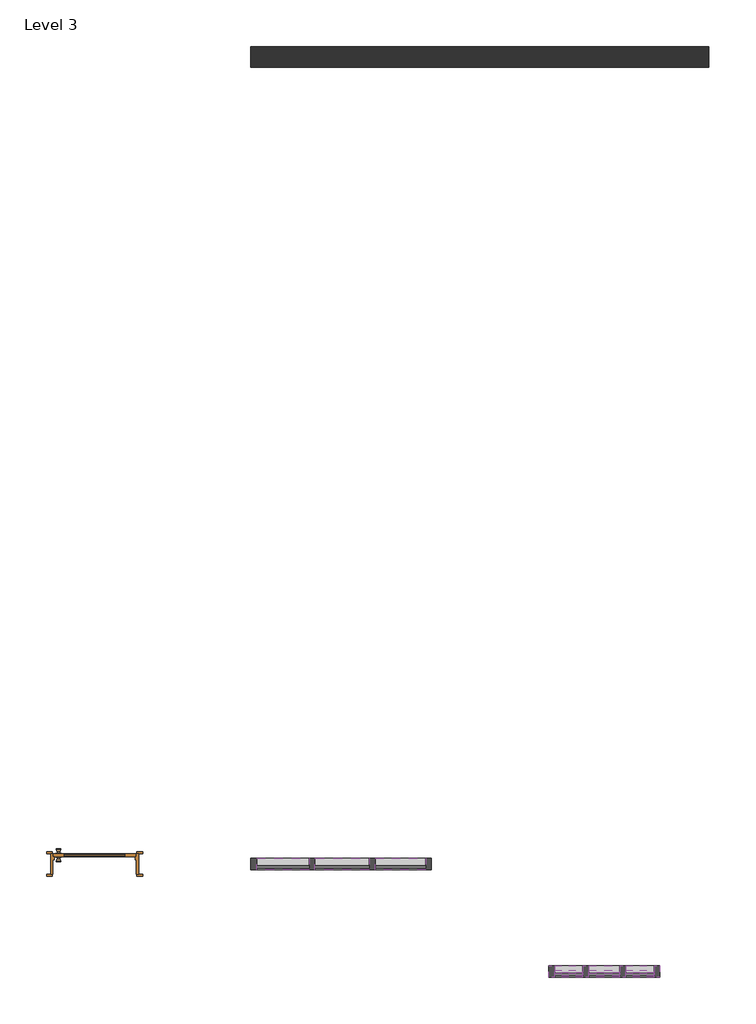
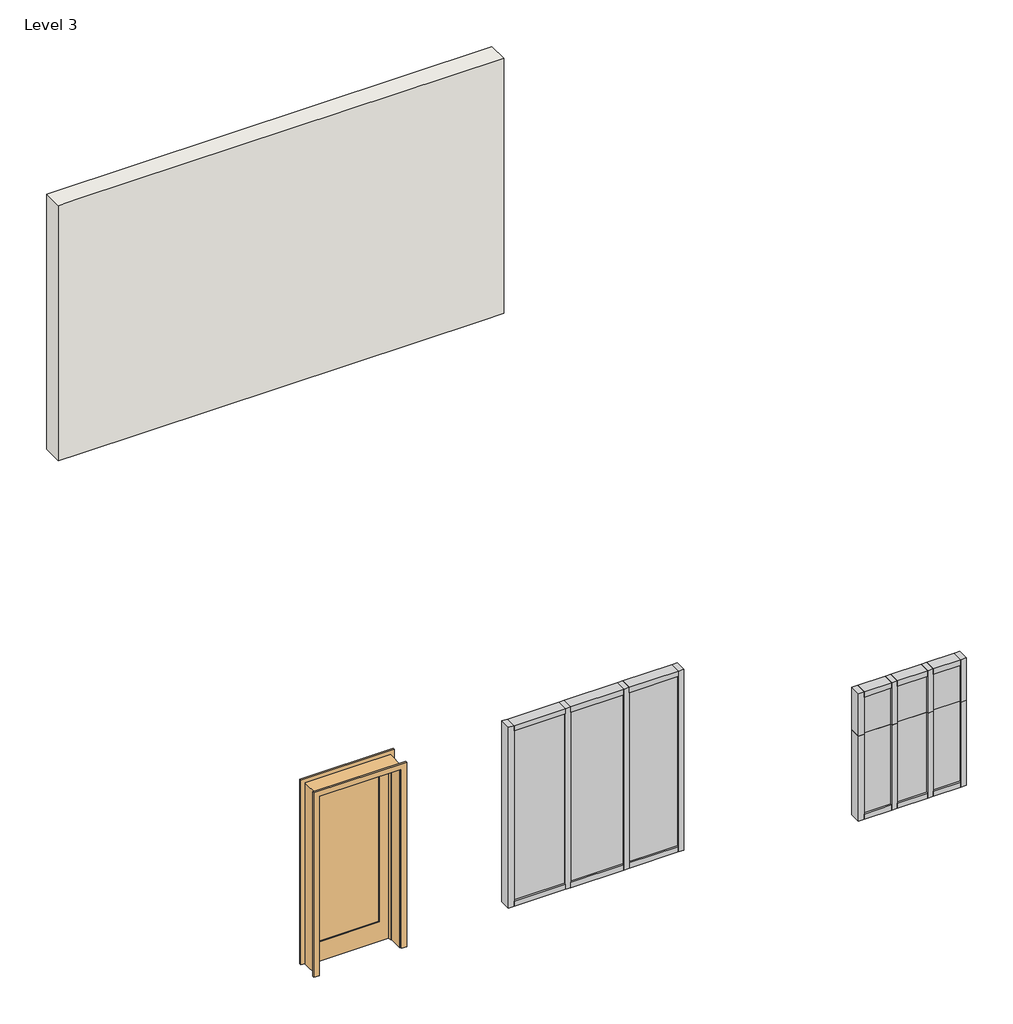
# One storey, incomplete: 27 members, 9 plates, 1 door, 1 wall.
"""IFC4 building model written with IfcOpenShell, lengths in millimetres."""

from ifc_helpers import new_model, si_unit, origin, place, context, project, spatial, faceted_brep, transform, mapped, element, save
from components import door_3b97b8e7, member_6c57b699, member_2c71ef08, member_5ad95953, member_f92b8aa2, member_ff1b7d8f, member_90750a43, member_7fd687a9, member_8e09d03a, member_c08f7e50, member_830eb86c, member_fb65e0d5, member_73c075c8, member_a400357f, system_panel_glazed_0360dae9, system_panel_glazed_809156e5, system_panel_glazed_ff0761ce, system_panel_glazed_bfcc9025, system_panel_glazed_b4fc352e, system_panel_glazed_a8841a5f, system_panel_glazed_4c4e158e

model = new_model("IFC4")

# Units and contexts
model_context = context("Model", 3, world=origin())
ifc_project = project(units=[si_unit("LENGTHUNIT", "METRE", prefix="MILLI")], contexts=[model_context])

# Site, building, storey
site = spatial("IfcSite", under=ifc_project)
building = spatial("IfcBuilding", under=site)
storey = spatial("IfcBuildingStorey", under=building, Name="Level 3", Elevation=3200.4)

# Door
placement = place(None, origin())
door_shape = door_3b97b8e7(model_context)
element("IfcDoor", 1, ObjectType="Door-Interior-Single-1_Panel-Wood : 36\" x 84\"", at=placement, inside=storey, context=model_context, shape_type="MappedRepresentation", body=[
    mapped(door_shape, transform((-5311.1915113, 1605.7349631, 3200.4), x_axis=(1.0, 0.0, 0.0), y_axis=(0.0, 1.0, 0.0), z_axis=(0.0, 0.0, 1.0))),
])

# Members
member_shape = member_6c57b699(model_context)
element("IfcMember", 2, ObjectType="Rectangular Mullion : 1\" Square", at=placement, inside=storey, context=model_context, shape_type="MappedRepresentation", body=[
    mapped(member_shape, transform((111.7084887, 421.4599631, 4826.0), x_axis=(0.0, 0.0, 1.0), y_axis=(0.0, 1.0, 0.0), z_axis=(-1.0, 0.0, 0.0))),
])
member_2_shape = member_2c71ef08(model_context)
element("IfcMember", 3, ObjectType="Rectangular Mullion : 1\" Square", at=placement, inside=storey, context=model_context, shape_type="MappedRepresentation", body=[
    mapped(member_2_shape, transform((-262.9415113, 421.4599631, 4826.0), x_axis=(0.0, 0.0, 1.0), y_axis=(0.0, 1.0, 0.0), z_axis=(-1.0, 0.0, 0.0))),
])
element("IfcMember", 4, ObjectType="Rectangular Mullion : 1\" Square", at=placement, inside=storey, context=model_context, shape_type="MappedRepresentation", body=[
    mapped(member_2_shape, transform((518.1084887, 421.4599631, 4826.0), x_axis=(0.0, 0.0, 1.0), y_axis=(0.0, 1.0, 0.0), z_axis=(-1.0, 0.0, 0.0))),
])
member_3_shape = member_5ad95953(model_context)
element("IfcMember", 5, ObjectType="Rectangular Mullion : 2.5\" x 5\" rectangular", at=placement, inside=storey, context=model_context, shape_type="MappedRepresentation", body=[
    mapped(member_3_shape, transform((-262.9415113, 421.4599631, 5334.0), x_axis=(0.0, 0.0, 1.0), y_axis=(0.0, 1.0, 0.0), z_axis=(-1.0, 0.0, 0.0))),
])
element("IfcMember", 6, ObjectType="Rectangular Mullion : 2.5\" x 5\" rectangular", at=placement, inside=storey, context=model_context, shape_type="MappedRepresentation", body=[
    mapped(member_3_shape, transform((518.1084887, 421.4599631, 5334.0), x_axis=(0.0, 0.0, 1.0), y_axis=(0.0, 1.0, 0.0), z_axis=(-1.0, 0.0, 0.0))),
])
element("IfcMember", 7, ObjectType="Rectangular Mullion : 2.5\" x 5\" rectangular", at=placement, inside=storey, context=model_context, shape_type="MappedRepresentation", body=[
    mapped(member_3_shape, transform((829.2584887, 421.4599631, 3810.0), x_axis=(0.0, 0.0, -1.0), y_axis=(0.0, 1.0, 0.0), z_axis=(1.0, 0.0, 0.0))),
])
element("IfcMember", 8, ObjectType="Rectangular Mullion : 2.5\" x 5\" rectangular", at=placement, inside=storey, context=model_context, shape_type="MappedRepresentation", body=[
    mapped(member_3_shape, transform((48.2084887, 421.4599631, 3810.0), x_axis=(0.0, 0.0, -1.0), y_axis=(0.0, 1.0, 0.0), z_axis=(1.0, 0.0, 0.0))),
])
member_4_shape = member_f92b8aa2(model_context)
element("IfcMember", 9, ObjectType="Rectangular Mullion : 2.5\" x 5\" rectangular", at=placement, inside=storey, context=model_context, shape_type="MappedRepresentation", body=[
    mapped(member_4_shape, transform((79.9584887, 421.4599631, 3810.0), x_axis=(-1.0, 0.0, 0.0), y_axis=(0.0, 1.0, 0.0), z_axis=(0.0, 0.0, -1.0))),
])
element("IfcMember", 10, ObjectType="Rectangular Mullion : 2.5\" x 5\" rectangular", at=placement, inside=storey, context=model_context, shape_type="MappedRepresentation", body=[
    mapped(member_4_shape, transform((486.3584887, 421.4599631, 3810.0), x_axis=(-1.0, 0.0, 0.0), y_axis=(0.0, 1.0, 0.0), z_axis=(0.0, 0.0, -1.0))),
])
member_5_shape = member_ff1b7d8f(model_context)
element("IfcMember", 11, ObjectType="Rectangular Mullion : 2.5\" x 5\" rectangular", at=placement, inside=storey, context=model_context, shape_type="MappedRepresentation", body=[
    mapped(member_5_shape, transform((454.6084887, 421.4599631, 3810.0), x_axis=(0.0, 0.0, -1.0), y_axis=(0.0, 1.0, 0.0), z_axis=(1.0, 0.0, 0.0))),
])
element("IfcMember", 12, ObjectType="Rectangular Mullion : 2.5\" x 5\" rectangular", at=placement, inside=storey, context=model_context, shape_type="MappedRepresentation", body=[
    mapped(member_5_shape, transform((111.7084887, 421.4599631, 5334.0), x_axis=(0.0, 0.0, 1.0), y_axis=(0.0, 1.0, 0.0), z_axis=(-1.0, 0.0, 0.0))),
])
member_6_shape = member_90750a43(model_context)
element("IfcMember", 13, ObjectType="Rectangular Mullion : 2.5\" x 5\" rectangular", at=placement, inside=storey, context=model_context, shape_type="MappedRepresentation", body=[
    mapped(member_6_shape, transform((79.9584887, 421.4599631, 4826.0), x_axis=(-1.0, 0.0, 0.0), y_axis=(0.0, 1.0, 0.0), z_axis=(0.0, 0.0, -1.0))),
])
element("IfcMember", 14, ObjectType="Rectangular Mullion : 2.5\" x 5\" rectangular", at=placement, inside=storey, context=model_context, shape_type="MappedRepresentation", body=[
    mapped(member_6_shape, transform((486.3584887, 421.4599631, 4826.0), x_axis=(-1.0, 0.0, 0.0), y_axis=(0.0, 1.0, 0.0), z_axis=(0.0, 0.0, -1.0))),
])
member_7_shape = member_7fd687a9(model_context)
element("IfcMember", 15, ObjectType="Rectangular Mullion : 2.5\" x 5\" rectangular", at=placement, inside=storey, context=model_context, shape_type="MappedRepresentation", body=[
    mapped(member_7_shape, transform((892.7584887, 421.4599631, 5334.0), x_axis=(1.0, 0.0, 0.0), y_axis=(0.0, 1.0, 0.0), z_axis=(0.0, 0.0, 1.0))),
])
member_8_shape = member_8e09d03a(model_context)
element("IfcMember", 16, ObjectType="Rectangular Mullion : 2.5\" x 5\" rectangular", at=placement, inside=storey, context=model_context, shape_type="MappedRepresentation", body=[
    mapped(member_8_shape, transform((-326.4415113, 421.4599631, 3810.0), x_axis=(-1.0, 0.0, 0.0), y_axis=(0.0, 1.0, 0.0), z_axis=(0.0, 0.0, -1.0))),
])
element("IfcMember", 17, ObjectType="Rectangular Mullion : 2.5\" x 5\" rectangular", at=placement, inside=storey, context=model_context, shape_type="MappedRepresentation", body=[
    mapped(member_7_shape, transform((-326.4415113, 421.4599631, 4826.0), x_axis=(-1.0, 0.0, 0.0), y_axis=(0.0, 1.0, 0.0), z_axis=(0.0, 0.0, -1.0))),
])
element("IfcMember", 18, ObjectType="Rectangular Mullion : 2.5\" x 5\" rectangular", at=placement, inside=storey, context=model_context, shape_type="MappedRepresentation", body=[
    mapped(member_8_shape, transform((892.7584887, 421.4599631, 4826.0), x_axis=(1.0, 0.0, 0.0), y_axis=(0.0, 1.0, 0.0), z_axis=(0.0, 0.0, 1.0))),
])
member_9_shape = member_c08f7e50(model_context)
element("IfcMember", 19, ObjectType="Rectangular Mullion : 2.5\" x 5\" rectangular", at=placement, inside=storey, context=model_context, shape_type="MappedRepresentation", body=[
    mapped(member_9_shape, transform((-1615.4915113, 1602.5599631, 5359.4), x_axis=(1.0, 0.0, 0.0), y_axis=(0.0, 1.0, 0.0), z_axis=(0.0, 0.0, 1.0))),
])
element("IfcMember", 20, ObjectType="Rectangular Mullion : 2.5\" x 5\" rectangular", at=placement, inside=storey, context=model_context, shape_type="MappedRepresentation", body=[
    mapped(member_9_shape, transform((-3596.6915113, 1602.5599631, 3200.4), x_axis=(-1.0, 0.0, 0.0), y_axis=(0.0, 1.0, 0.0), z_axis=(0.0, 0.0, -1.0))),
])
member_10_shape = member_830eb86c(model_context)
element("IfcMember", 21, ObjectType="Rectangular Mullion : 2.5\" x 5\" rectangular", at=placement, inside=storey, context=model_context, shape_type="MappedRepresentation", body=[
    mapped(member_10_shape, transform((-3533.1915113, 1602.5599631, 5359.4), x_axis=(0.0, 0.0, 1.0), y_axis=(0.0, 1.0, 0.0), z_axis=(-1.0, 0.0, 0.0))),
])
element("IfcMember", 22, ObjectType="Rectangular Mullion : 2.5\" x 5\" rectangular", at=placement, inside=storey, context=model_context, shape_type="MappedRepresentation", body=[
    mapped(member_10_shape, transform((-2955.3415113, 1602.5599631, 3200.4), x_axis=(0.0, 0.0, -1.0), y_axis=(0.0, 1.0, 0.0), z_axis=(1.0, 0.0, 0.0))),
])
member_11_shape = member_fb65e0d5(model_context)
element("IfcMember", 23, ObjectType="Rectangular Mullion : 2.5\" x 5\" rectangular", at=placement, inside=storey, context=model_context, shape_type="MappedRepresentation", body=[
    mapped(member_11_shape, transform((-2923.5915113, 1602.5599631, 3200.4), x_axis=(-1.0, 0.0, 0.0), y_axis=(0.0, 1.0, 0.0), z_axis=(0.0, 0.0, -1.0))),
])
element("IfcMember", 24, ObjectType="Rectangular Mullion : 2.5\" x 5\" rectangular", at=placement, inside=storey, context=model_context, shape_type="MappedRepresentation", body=[
    mapped(member_11_shape, transform((-2263.1915113, 1602.5599631, 3200.4), x_axis=(-1.0, 0.0, 0.0), y_axis=(0.0, 1.0, 0.0), z_axis=(0.0, 0.0, -1.0))),
])
member_12_shape = member_73c075c8(model_context)
element("IfcMember", 25, ObjectType="Rectangular Mullion : 2.5\" x 5\" rectangular", at=placement, inside=storey, context=model_context, shape_type="MappedRepresentation", body=[
    mapped(member_12_shape, transform((-1678.9915113, 1602.5599631, 3200.4), x_axis=(0.0, 0.0, -1.0), y_axis=(0.0, 1.0, 0.0), z_axis=(1.0, 0.0, 0.0))),
])
member_13_shape = member_a400357f(model_context)
element("IfcMember", 26, ObjectType="Rectangular Mullion : 2.5\" x 5\" rectangular", at=placement, inside=storey, context=model_context, shape_type="MappedRepresentation", body=[
    mapped(member_13_shape, transform((-2294.9415113, 1602.5599631, 3200.4), x_axis=(0.0, 0.0, -1.0), y_axis=(0.0, 1.0, 0.0), z_axis=(1.0, 0.0, 0.0))),
])
element("IfcMember", 27, ObjectType="Rectangular Mullion : 2.5\" x 5\" rectangular", at=placement, inside=storey, context=model_context, shape_type="MappedRepresentation", body=[
    mapped(member_13_shape, transform((-2891.8415113, 1602.5599631, 5359.4), x_axis=(0.0, 0.0, 1.0), y_axis=(0.0, 1.0, 0.0), z_axis=(-1.0, 0.0, 0.0))),
])
element("IfcMember", 28, ObjectType="Rectangular Mullion : 2.5\" x 5\" rectangular", at=placement, inside=storey, context=model_context, shape_type="MappedRepresentation", body=[
    mapped(member_12_shape, transform((-2231.4415113, 1602.5599631, 5359.4), x_axis=(0.0, 0.0, 1.0), y_axis=(0.0, 1.0, 0.0), z_axis=(-1.0, 0.0, 0.0))),
])

# Plates
system_panel_glazed_shape = system_panel_glazed_0360dae9(model_context)
element("IfcPlate", 29, ObjectType="System Panel : Glazed", at=placement, inside=storey, context=model_context, shape_type="MappedRepresentation", body=[
    mapped(system_panel_glazed_shape, transform((673.6834887, 421.4599631, 3873.5), x_axis=(-1.0, 0.0, 0.0), y_axis=(0.0, -1.0, 0.0), z_axis=(0.0, 0.0, 1.0))),
])
element("IfcPlate", 30, ObjectType="System Panel : Glazed", at=placement, inside=storey, context=model_context, shape_type="MappedRepresentation", body=[
    mapped(system_panel_glazed_shape, transform((-107.3665113, 421.4599631, 3873.5), x_axis=(-1.0, 0.0, 0.0), y_axis=(0.0, -1.0, 0.0), z_axis=(0.0, 0.0, 1.0))),
])
system_panel_glazed_2_shape = system_panel_glazed_809156e5(model_context)
element("IfcPlate", 31, ObjectType="System Panel : Glazed", at=placement, inside=storey, context=model_context, shape_type="MappedRepresentation", body=[
    mapped(system_panel_glazed_2_shape, transform((283.1584887, 421.4599631, 3873.5), x_axis=(-1.0, 0.0, 0.0), y_axis=(0.0, -1.0, 0.0), z_axis=(0.0, 0.0, 1.0))),
])
system_panel_glazed_3_shape = system_panel_glazed_ff0761ce(model_context)
element("IfcPlate", 32, ObjectType="System Panel : Glazed", at=placement, inside=storey, context=model_context, shape_type="MappedRepresentation", body=[
    mapped(system_panel_glazed_3_shape, transform((673.6834887, 421.4599631, 4826.0), x_axis=(-1.0, 0.0, 0.0), y_axis=(0.0, -1.0, 0.0), z_axis=(0.0, 0.0, 1.0))),
])
element("IfcPlate", 33, ObjectType="System Panel : Glazed", at=placement, inside=storey, context=model_context, shape_type="MappedRepresentation", body=[
    mapped(system_panel_glazed_3_shape, transform((-107.3665113, 421.4599631, 4826.0), x_axis=(-1.0, 0.0, 0.0), y_axis=(0.0, -1.0, 0.0), z_axis=(0.0, 0.0, 1.0))),
])
system_panel_glazed_4_shape = system_panel_glazed_bfcc9025(model_context)
element("IfcPlate", 34, ObjectType="System Panel : Glazed", at=placement, inside=storey, context=model_context, shape_type="MappedRepresentation", body=[
    mapped(system_panel_glazed_4_shape, transform((283.1584887, 421.4599631, 4826.0), x_axis=(-1.0, 0.0, 0.0), y_axis=(0.0, -1.0, 0.0), z_axis=(0.0, 0.0, 1.0))),
])
system_panel_glazed_5_shape = system_panel_glazed_b4fc352e(model_context)
element("IfcPlate", 35, ObjectType="System Panel : Glazed", at=placement, inside=storey, context=model_context, shape_type="MappedRepresentation", body=[
    mapped(system_panel_glazed_5_shape, transform((-3244.2665113, 1602.5599631, 3263.9), x_axis=(-1.0, 0.0, 0.0), y_axis=(0.0, -1.0, 0.0), z_axis=(0.0, 0.0, 1.0))),
])
system_panel_glazed_6_shape = system_panel_glazed_a8841a5f(model_context)
element("IfcPlate", 36, ObjectType="System Panel : Glazed", at=placement, inside=storey, context=model_context, shape_type="MappedRepresentation", body=[
    mapped(system_panel_glazed_6_shape, transform((-1955.2165113, 1602.5599631, 3263.9), x_axis=(-1.0, 0.0, 0.0), y_axis=(0.0, -1.0, 0.0), z_axis=(0.0, 0.0, 1.0))),
])
system_panel_glazed_7_shape = system_panel_glazed_4c4e158e(model_context)
element("IfcPlate", 37, ObjectType="System Panel : Glazed", at=placement, inside=storey, context=model_context, shape_type="MappedRepresentation", body=[
    mapped(system_panel_glazed_7_shape, transform((-2593.3915113, 1602.5599631, 3263.9), x_axis=(-1.0, 0.0, 0.0), y_axis=(0.0, -1.0, 0.0), z_axis=(0.0, 0.0, 1.0))),
])

# Wall
element("IfcWall", 38, ObjectType="9\" wall", at=placement, inside=storey, context=model_context, shape_type="Brep", body=[
    faceted_brep([(1432.5084887, 10575.1099631, 3200.4), (-3596.6915113, 10575.1099631, 3200.4), (-3596.6915113, 10575.1099631, 6248.4), (1432.5084887, 10575.1099631, 6248.4), (1432.5084887, 10346.5099631, 3200.4), (1432.5084887, 10346.5099631, 6001.9502231), (1432.5084887, 10346.5099631, 6248.4), (-3368.0915113, 10346.5099631, 6248.4), (-3596.6915113, 10346.5099631, 6248.4), (-3596.6915113, 10346.5099631, 3200.4), (-3368.0915113, 10346.5099631, 3200.4), (1203.9084887, 10346.5099631, 3200.4)], [[[0, 1, 2, 3]], [[4, 5, 6, 7, 8, 9, 10, 11]], [[1, 0, 4, 11, 10, 9]], [[3, 2, 8, 7, 6]], [[0, 3, 6, 5, 4]], [[2, 1, 9, 8]]]),
])

save(model, "model.ifc")

# Revit data of these elements
# Type "Door-Interior-Single-1_Panel-Wood : 36\" x 84\""
#   Type Mark = "8"
#   Assembly Code = "C1020300"
#   Analytic Construction = "Wooden"
#   Top Rail = 0' - 4 11/16"
#   Thickness = 0' - 1 3/8"
#   Thermal Resistance (R) = 2.5876 (h·ft²·°F)/BTU
#   Swing Angle [instance default] = 90.00°
#   Stiles = 0' - 4 3/4"
#   Rough Width = 3' - 2"
#   Rough Height = 7' - 1"
#   Height = 7' - 0"
#   Width = 3' - 0"
#   Heat Transfer Coefficient (U) = 0.3865 BTU/(h·ft²·°F)
#   Bottom Rail = 0' - 9 1/8"
#   Trim Material = Cherry
#   Panel Material = Cherry
#   Frame Material = Cherry
#   Door Handle Material = Aluminum
#   Visual Light Transmittance = 0
#   Solar Heat Gain Coefficient = 0
#   Wall Closure = (empty or 0)
#   Function = (empty or 0)
# Type "Rectangular Mullion : 1\" Square"
#   built-in parameter 1007304 = 0.0833333 (stored number, unit not read)
#   built-in parameter 1007301 = 0.0416667 (stored number, unit not read)
#   built-in parameter 1007300 = 0.0416667 (stored number, unit not read)
# Type "Rectangular Mullion : 2.5\" x 5\" rectangular"
#   built-in parameter 1007304 = 0.416667 (stored number, unit not read)
#   built-in parameter 1007301 = 0.104167 (stored number, unit not read)
#   built-in parameter 1007300 = 0.104167 (stored number, unit not read)
# Type "System Panel : Glazed"
#   Construction Type Id = "GSP4R"
#   Analytic Construction = "1/8 in Pilkington single glazing"
#   Visual Light Transmittance = 0.9
#   Solar Heat Gain Coefficient = 0.86
#   Heat Transfer Coefficient (U) = 1.18115 BTU/(h·ft²·°F)
#   Define Thermal Properties by = 1
# Type "9\" wall"
#   Assembly Code = "B2010"
#   Layers, outside or top first: 0' - 9" "Laminate, Ivory, Matte" (function 1)
# Element 1 (IfcDoor, "Door-Interior-Single-1_Panel-Wood : 36\" x 84\"")
#   Swing Angle = 90.00°
#   Phase Created = New Construction
#   Materials on its faces: "Cherry", "Aluminum"
# Elements 2, 3, 4 (IfcMember, "Rectangular Mullion : 1\" Square")
#   Phase Created = New Construction
# Elements 5, 6, 7, 8, 9, 10, 11, 12, 13, 14, 15, 16, 17, 18, 19, 20, 21, 22, 23, 24, 25, 26, 27, 28 (IfcMember, "Rectangular Mullion : 2.5\" x 5\" rectangular")
#   Phase Created = New Construction
# Elements 29, 30, 31, 32, 33, 34, 35, 36, 37 (IfcPlate, "System Panel : Glazed")
#   Phase Created = New Construction
#   Materials on its faces: "Glass"
# Element 38 (IfcWall, "9\" wall")
#   Top Offset = 10' - 0"
#   Base Offset = 0' - 0"
#   wall height = 10' - 0"
#   Phase Created = New Construction
#   Base Constraint = Level 3
#   Top Constraint = Level 3
#   Materials on its faces: "Laminate, Ivory, Matte"
# Materials
#   "Cherry": class "Wood", colour RGB 226 177 128, transparency 0, Description = "Prunus Serotina", Cost = 0
#   "Aluminum": class "Metal", colour RGB 247 247 247, transparency 0, Description = "Aluminum 6061", Cost = 0
#   "Laminate, Ivory, Matte": class "Plastic", colour RGB 247 247 239, transparency 0, Description = "Plastic Laminate - Ivory, Matte", Cost = 0
#   "Glass": class "Glass", colour RGB 0 128 192, transparency 0.75, Description = "Soda Lime Glass", Cost = 0
